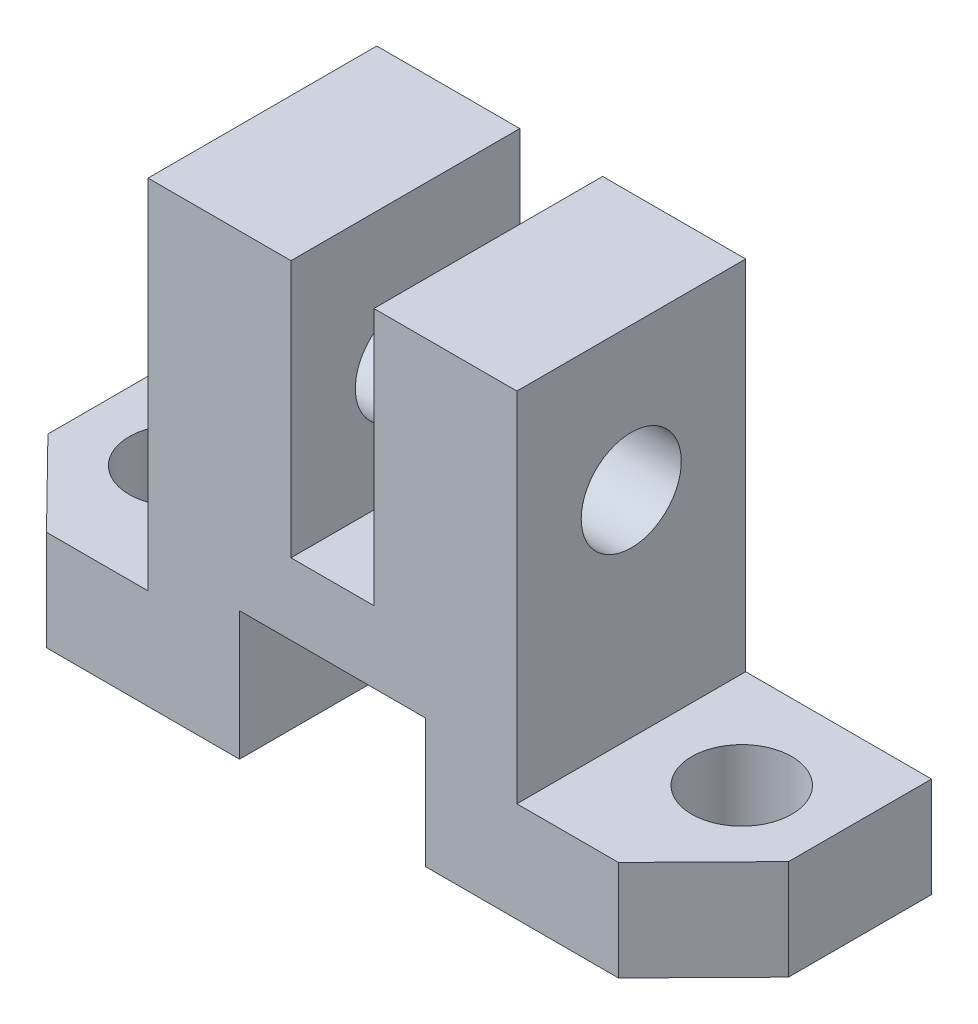
ISO-10303-21;
HEADER;
FILE_DESCRIPTION(('STEP AP214'),'2;1');
FILE_NAME('part.step','',(''),(''),'','','');
FILE_SCHEMA(('AUTOMOTIVE_DESIGN { 1 0 10303 214 1 1 1 1 }'));
ENDSEC;
DATA;
#1=APPLICATION_CONTEXT('core data for automotive mechanical design processes');
#2=APPLICATION_PROTOCOL_DEFINITION('international standard','automotive_design',2000,#1);
#3=PRODUCT_CONTEXT('',#1,'mechanical');
#4=PRODUCT('Part','Part','',(#3));
#5=PRODUCT_RELATED_PRODUCT_CATEGORY('part','',(#4));
#6=PRODUCT_DEFINITION_FORMATION('','',#4);
#7=PRODUCT_DEFINITION_CONTEXT('part definition',#1,'design');
#8=PRODUCT_DEFINITION('design','',#6,#7);
#9=PRODUCT_DEFINITION_SHAPE('','',#8);
#10=(LENGTH_UNIT() NAMED_UNIT(*) SI_UNIT(.MILLI.,.METRE.));
#11=(NAMED_UNIT(*) PLANE_ANGLE_UNIT() SI_UNIT($,.RADIAN.));
#12=(NAMED_UNIT(*) SI_UNIT($,.STERADIAN.) SOLID_ANGLE_UNIT());
#13=UNCERTAINTY_MEASURE_WITH_UNIT(LENGTH_MEASURE(1.E-05),#10,'distance_accuracy_value','');
#14=(GEOMETRIC_REPRESENTATION_CONTEXT(3) GLOBAL_UNCERTAINTY_ASSIGNED_CONTEXT((#13)) GLOBAL_UNIT_ASSIGNED_CONTEXT((#10,
#11,#12)) REPRESENTATION_CONTEXT('',''));
#15=CARTESIAN_POINT('',(0.,0.,0.));
#16=DIRECTION('',(0.,0.,1.));
#17=DIRECTION('',(1.,0.,0.));
#18=AXIS2_PLACEMENT_3D('',#15,#16,#17);
#19=CARTESIAN_POINT('',(-51.7969552583166,7.,2.19710608259383));
#20=DIRECTION('',(0.,0.,1.));
#21=DIRECTION('',(1.,0.,0.));
#22=AXIS2_PLACEMENT_3D('',#19,#20,#21);
#23=PLANE('',#22);
#24=DIRECTION('',(0.,-1.,0.));
#25=VECTOR('',#24,1.);
#26=CARTESIAN_POINT('',(-19.3984776291583,7.,2.19710608259383));
#27=LINE('',#26,#25);
#28=CARTESIAN_POINT('',(-19.3984776291583,9.,2.19710608259382));
#29=VERTEX_POINT('',#28);
#30=CARTESIAN_POINT('',(-19.3984776291583,0.,2.19710608259382));
#31=VERTEX_POINT('',#30);
#32=EDGE_CURVE('E190',#29,#31,#27,.T.);
#33=ORIENTED_EDGE('',*,*,#32,.F.);
#34=DIRECTION('',(1.,0.,0.));
#35=VECTOR('',#34,1.);
#36=CARTESIAN_POINT('',(-51.7969552583166,9.,2.19710608259383));
#37=LINE('',#36,#35);
#38=CARTESIAN_POINT('',(-32.3984776291583,9.,2.19710608259382));
#39=VERTEX_POINT('',#38);
#40=EDGE_CURVE('E186',#39,#29,#37,.T.);
#41=ORIENTED_EDGE('',*,*,#40,.F.);
#42=DIRECTION('',(0.,1.,0.));
#43=VECTOR('',#42,1.);
#44=CARTESIAN_POINT('',(-32.3984776291583,7.,2.19710608259383));
#45=LINE('',#44,#43);
#46=CARTESIAN_POINT('',(-32.3984776291583,0.,2.19710608259382));
#47=VERTEX_POINT('',#46);
#48=EDGE_CURVE('E172',#47,#39,#45,.T.);
#49=ORIENTED_EDGE('',*,*,#48,.F.);
#50=DIRECTION('',(-1.,0.,0.));
#51=VECTOR('',#50,1.);
#52=CARTESIAN_POINT('',(-51.7969552583166,0.,2.19710608259383));
#53=LINE('',#52,#51);
#54=CARTESIAN_POINT('',(-51.7969552583166,0.,2.19710608259383));
#55=VERTEX_POINT('',#54);
#56=EDGE_CURVE('E251',#47,#55,#53,.T.);
#57=ORIENTED_EDGE('',*,*,#56,.T.);
#58=DIRECTION('',(0.,-1.,0.));
#59=VECTOR('',#58,1.);
#60=CARTESIAN_POINT('',(-51.7969552583166,7.,2.19710608259383));
#61=LINE('',#60,#59);
#62=CARTESIAN_POINT('',(-51.7969552583166,7.,2.19710608259383));
#63=VERTEX_POINT('',#62);
#64=EDGE_CURVE('E298',#63,#55,#61,.T.);
#65=ORIENTED_EDGE('',*,*,#64,.F.);
#66=DIRECTION('',(-1.,0.,0.));
#67=VECTOR('',#66,1.);
#68=CARTESIAN_POINT('',(-51.7969552583166,7.,2.19710608259383));
#69=LINE('',#68,#67);
#70=CARTESIAN_POINT('',(-38.7969552583166,7.,2.19710608259383));
#71=VERTEX_POINT('',#70);
#72=EDGE_CURVE('E260',#71,#63,#69,.T.);
#73=ORIENTED_EDGE('',*,*,#72,.F.);
#74=DIRECTION('',(0.,-1.,0.));
#75=VECTOR('',#74,1.);
#76=CARTESIAN_POINT('',(-38.7969552583166,32.,2.19710608259383));
#77=LINE('',#76,#75);
#78=CARTESIAN_POINT('',(-38.7969552583166,32.,2.19710608259383));
#79=VERTEX_POINT('',#78);
#80=EDGE_CURVE('E240',#79,#71,#77,.T.);
#81=ORIENTED_EDGE('',*,*,#80,.F.);
#82=DIRECTION('',(-1.,0.,0.));
#83=VECTOR('',#82,1.);
#84=CARTESIAN_POINT('',(-38.7969552583166,32.,2.19710608259383));
#85=LINE('',#84,#83);
#86=CARTESIAN_POINT('',(-28.7969552583166,32.,2.19710608259382));
#87=VERTEX_POINT('',#86);
#88=EDGE_CURVE('E225',#87,#79,#85,.T.);
#89=ORIENTED_EDGE('',*,*,#88,.F.);
#90=DIRECTION('',(0.,1.,0.));
#91=VECTOR('',#90,1.);
#92=CARTESIAN_POINT('',(-28.7969552583166,7.,2.19710608259383));
#93=LINE('',#92,#91);
#94=CARTESIAN_POINT('',(-28.7969552583166,14.,2.19710608259382));
#95=VERTEX_POINT('',#94);
#96=EDGE_CURVE('E211',#95,#87,#93,.T.);
#97=ORIENTED_EDGE('',*,*,#96,.F.);
#98=DIRECTION('',(-1.,0.,0.));
#99=VECTOR('',#98,1.);
#100=CARTESIAN_POINT('',(-51.7969552583166,14.,2.19710608259383));
#101=LINE('',#100,#99);
#102=CARTESIAN_POINT('',(-23.,14.,2.19710608259382));
#103=VERTEX_POINT('',#102);
#104=EDGE_CURVE('E213',#103,#95,#101,.T.);
#105=ORIENTED_EDGE('',*,*,#104,.F.);
#106=DIRECTION('',(0.,-1.,0.));
#107=VECTOR('',#106,1.);
#108=CARTESIAN_POINT('',(-23.,7.00000000000001,2.19710608259383));
#109=LINE('',#108,#107);
#110=CARTESIAN_POINT('',(-23.,32.,2.19710608259382));
#111=VERTEX_POINT('',#110);
#112=EDGE_CURVE('E206',#111,#103,#109,.T.);
#113=ORIENTED_EDGE('',*,*,#112,.F.);
#114=CARTESIAN_POINT('',(-13.,32.,2.19710608259382));
#115=VERTEX_POINT('',#114);
#116=EDGE_CURVE('E223',#115,#111,#85,.T.);
#117=ORIENTED_EDGE('',*,*,#116,.F.);
#118=DIRECTION('',(0.,-1.,0.));
#119=VECTOR('',#118,1.);
#120=CARTESIAN_POINT('',(-13.,32.,2.19710608259382));
#121=LINE('',#120,#119);
#122=CARTESIAN_POINT('',(-13.,7.,2.19710608259382));
#123=VERTEX_POINT('',#122);
#124=EDGE_CURVE('E239',#115,#123,#121,.T.);
#125=ORIENTED_EDGE('',*,*,#124,.T.);
#126=CARTESIAN_POINT('',(0.,7.,2.19710608259383));
#127=VERTEX_POINT('',#126);
#128=EDGE_CURVE('E253',#127,#123,#69,.T.);
#129=ORIENTED_EDGE('',*,*,#128,.F.);
#130=DIRECTION('',(0.,-1.,0.));
#131=VECTOR('',#130,1.);
#132=CARTESIAN_POINT('',(0.,7.,2.19710608259383));
#133=LINE('',#132,#131);
#134=CARTESIAN_POINT('',(0.,0.,2.19710608259383));
#135=VERTEX_POINT('',#134);
#136=EDGE_CURVE('E268',#127,#135,#133,.T.);
#137=ORIENTED_EDGE('',*,*,#136,.T.);
#138=EDGE_CURVE('E267',#135,#31,#53,.T.);
#139=ORIENTED_EDGE('',*,*,#138,.T.);
#140=EDGE_LOOP('',(#33,#41,#49,#57,#65,#73,#81,#89,#97,#105,#113,#117,#125,#129,#137,#139));
#141=FACE_BOUND('',#140,.T.);
#142=ADVANCED_FACE('F39',(#141),#23,.F.);
#143=CARTESIAN_POINT('',(-45.8984776291583,7.,18.1971060825938));
#144=DIRECTION('',(0.,0.,-1.));
#145=DIRECTION('',(-1.,0.,0.));
#146=AXIS2_PLACEMENT_3D('',#143,#144,#145);
#147=PLANE('',#146);
#148=DIRECTION('',(0.,1.,0.));
#149=VECTOR('',#148,1.);
#150=CARTESIAN_POINT('',(-19.3984776291583,7.,18.1971060825938));
#151=LINE('',#150,#149);
#152=CARTESIAN_POINT('',(-19.3984776291583,0.,18.1971060825938));
#153=VERTEX_POINT('',#152);
#154=CARTESIAN_POINT('',(-19.3984776291583,9.,18.1971060825938));
#155=VERTEX_POINT('',#154);
#156=EDGE_CURVE('E185',#153,#155,#151,.T.);
#157=ORIENTED_EDGE('',*,*,#156,.F.);
#158=DIRECTION('',(1.,0.,0.));
#159=VECTOR('',#158,1.);
#160=CARTESIAN_POINT('',(-45.8984776291583,0.,18.1971060825938));
#161=LINE('',#160,#159);
#162=CARTESIAN_POINT('',(-5.89847762915829,0.,18.1971060825938));
#163=VERTEX_POINT('',#162);
#164=EDGE_CURVE('E276',#153,#163,#161,.T.);
#165=ORIENTED_EDGE('',*,*,#164,.T.);
#166=DIRECTION('',(0.,-1.,0.));
#167=VECTOR('',#166,1.);
#168=CARTESIAN_POINT('',(-5.89847762915829,7.,18.1971060825938));
#169=LINE('',#168,#167);
#170=CARTESIAN_POINT('',(-5.89847762915829,7.,18.1971060825938));
#171=VERTEX_POINT('',#170);
#172=EDGE_CURVE('E290',#171,#163,#169,.T.);
#173=ORIENTED_EDGE('',*,*,#172,.F.);
#174=DIRECTION('',(1.,0.,0.));
#175=VECTOR('',#174,1.);
#176=CARTESIAN_POINT('',(-45.8984776291583,7.,18.1971060825938));
#177=LINE('',#176,#175);
#178=CARTESIAN_POINT('',(-13.,7.,18.1971060825938));
#179=VERTEX_POINT('',#178);
#180=EDGE_CURVE('E265',#179,#171,#177,.T.);
#181=ORIENTED_EDGE('',*,*,#180,.F.);
#182=DIRECTION('',(0.,-1.,0.));
#183=VECTOR('',#182,1.);
#184=CARTESIAN_POINT('',(-13.,32.,18.1971060825938));
#185=LINE('',#184,#183);
#186=CARTESIAN_POINT('',(-13.,32.,18.1971060825938));
#187=VERTEX_POINT('',#186);
#188=EDGE_CURVE('E243',#187,#179,#185,.T.);
#189=ORIENTED_EDGE('',*,*,#188,.F.);
#190=DIRECTION('',(1.,0.,0.));
#191=VECTOR('',#190,1.);
#192=CARTESIAN_POINT('',(-13.,32.,18.1971060825938));
#193=LINE('',#192,#191);
#194=CARTESIAN_POINT('',(-23.,32.,18.1971060825938));
#195=VERTEX_POINT('',#194);
#196=EDGE_CURVE('E224',#195,#187,#193,.T.);
#197=ORIENTED_EDGE('',*,*,#196,.F.);
#198=DIRECTION('',(0.,1.,0.));
#199=VECTOR('',#198,1.);
#200=CARTESIAN_POINT('',(-23.,7.00000000000001,18.1971060825938));
#201=LINE('',#200,#199);
#202=CARTESIAN_POINT('',(-23.,14.,18.1971060825938));
#203=VERTEX_POINT('',#202);
#204=EDGE_CURVE('E64',#203,#195,#201,.T.);
#205=ORIENTED_EDGE('',*,*,#204,.F.);
#206=DIRECTION('',(1.,0.,0.));
#207=VECTOR('',#206,1.);
#208=CARTESIAN_POINT('',(-45.8984776291583,14.,18.1971060825938));
#209=LINE('',#208,#207);
#210=CARTESIAN_POINT('',(-28.7969552583166,14.,18.1971060825938));
#211=VERTEX_POINT('',#210);
#212=EDGE_CURVE('E310',#211,#203,#209,.T.);
#213=ORIENTED_EDGE('',*,*,#212,.F.);
#214=DIRECTION('',(0.,-1.,0.));
#215=VECTOR('',#214,1.);
#216=CARTESIAN_POINT('',(-28.7969552583166,7.,18.1971060825938));
#217=LINE('',#216,#215);
#218=CARTESIAN_POINT('',(-28.7969552583166,32.,18.1971060825938));
#219=VERTEX_POINT('',#218);
#220=EDGE_CURVE('E208',#219,#211,#217,.T.);
#221=ORIENTED_EDGE('',*,*,#220,.F.);
#222=CARTESIAN_POINT('',(-38.7969552583166,32.,18.1971060825938));
#223=VERTEX_POINT('',#222);
#224=EDGE_CURVE('E220',#223,#219,#193,.T.);
#225=ORIENTED_EDGE('',*,*,#224,.F.);
#226=DIRECTION('',(0.,-1.,0.));
#227=VECTOR('',#226,1.);
#228=CARTESIAN_POINT('',(-38.7969552583166,32.,18.1971060825938));
#229=LINE('',#228,#227);
#230=CARTESIAN_POINT('',(-38.7969552583166,7.,18.1971060825938));
#231=VERTEX_POINT('',#230);
#232=EDGE_CURVE('E230',#223,#231,#229,.T.);
#233=ORIENTED_EDGE('',*,*,#232,.T.);
#234=CARTESIAN_POINT('',(-45.8984776291583,7.,18.1971060825938));
#235=VERTEX_POINT('',#234);
#236=EDGE_CURVE('E264',#235,#231,#177,.T.);
#237=ORIENTED_EDGE('',*,*,#236,.F.);
#238=DIRECTION('',(0.,-1.,0.));
#239=VECTOR('',#238,1.);
#240=CARTESIAN_POINT('',(-45.8984776291583,7.,18.1971060825938));
#241=LINE('',#240,#239);
#242=CARTESIAN_POINT('',(-45.8984776291583,0.,18.1971060825938));
#243=VERTEX_POINT('',#242);
#244=EDGE_CURVE('E293',#235,#243,#241,.T.);
#245=ORIENTED_EDGE('',*,*,#244,.T.);
#246=CARTESIAN_POINT('',(-32.3984776291583,0.,18.1971060825938));
#247=VERTEX_POINT('',#246);
#248=EDGE_CURVE('E179',#243,#247,#161,.T.);
#249=ORIENTED_EDGE('',*,*,#248,.T.);
#250=DIRECTION('',(0.,-1.,0.));
#251=VECTOR('',#250,1.);
#252=CARTESIAN_POINT('',(-32.3984776291583,7.,18.1971060825938));
#253=LINE('',#252,#251);
#254=CARTESIAN_POINT('',(-32.3984776291583,9.,18.1971060825938));
#255=VERTEX_POINT('',#254);
#256=EDGE_CURVE('E52',#255,#247,#253,.T.);
#257=ORIENTED_EDGE('',*,*,#256,.F.);
#258=DIRECTION('',(-1.,0.,0.));
#259=VECTOR('',#258,1.);
#260=CARTESIAN_POINT('',(-45.8984776291583,9.,18.1971060825938));
#261=LINE('',#260,#259);
#262=EDGE_CURVE('E11',#155,#255,#261,.T.);
#263=ORIENTED_EDGE('',*,*,#262,.F.);
#264=EDGE_LOOP('',(#157,#165,#173,#181,#189,#197,#205,#213,#221,#225,#233,#237,#245,#249,#257,#263));
#265=FACE_BOUND('',#264,.T.);
#266=ADVANCED_FACE('F180',(#265),#147,.F.);
#267=CARTESIAN_POINT('',(0.,0.,0.));
#268=DIRECTION('',(0.,1.,0.));
#269=DIRECTION('',(0.,0.,1.));
#270=AXIS2_PLACEMENT_3D('',#267,#268,#269);
#271=PLANE('',#270);
#272=CARTESIAN_POINT('',(-6.25051200255727,0.,9.21864036847825));
#273=DIRECTION('',(0.,1.,0.));
#274=DIRECTION('',(0.,0.,1.));
#275=AXIS2_PLACEMENT_3D('',#272,#273,#274);
#276=CIRCLE('',#275,3.5);
#277=CARTESIAN_POINT('',(-6.25051200255727,0.,12.7186403684782));
#278=VERTEX_POINT('',#277);
#279=EDGE_CURVE('E246',#278,#278,#276,.F.);
#280=ORIENTED_EDGE('',*,*,#279,.F.);
#281=EDGE_LOOP('',(#280));
#282=FACE_BOUND('',#281,.T.);
#283=DIRECTION('',(0.,0.,1.));
#284=VECTOR('',#283,1.);
#285=CARTESIAN_POINT('',(-19.3984776291583,0.,0.));
#286=LINE('',#285,#284);
#287=EDGE_CURVE('E46',#31,#153,#286,.T.);
#288=ORIENTED_EDGE('',*,*,#287,.F.);
#289=ORIENTED_EDGE('',*,*,#138,.F.);
#290=DIRECTION('',(0.,0.,-1.));
#291=VECTOR('',#290,1.);
#292=CARTESIAN_POINT('',(0.,0.,12.1971060825938));
#293=LINE('',#292,#291);
#294=CARTESIAN_POINT('',(0.,0.,12.1971060825938));
#295=VERTEX_POINT('',#294);
#296=EDGE_CURVE('E282',#295,#135,#293,.T.);
#297=ORIENTED_EDGE('',*,*,#296,.F.);
#298=DIRECTION('',(0.701047956924281,0.,-0.713114129780284));
#299=VECTOR('',#298,1.);
#300=CARTESIAN_POINT('',(-5.89847762915829,0.,18.1971060825938));
#301=LINE('',#300,#299);
#302=EDGE_CURVE('E278',#163,#295,#301,.T.);
#303=ORIENTED_EDGE('',*,*,#302,.F.);
#304=ORIENTED_EDGE('',*,*,#164,.F.);
#305=EDGE_LOOP('',(#288,#289,#297,#303,#304));
#306=FACE_BOUND('',#305,.T.);
#307=ADVANCED_FACE('F324',(#282,#306),#271,.F.);
#308=CARTESIAN_POINT('',(-45.2969552583166,0.,9.51970674205226));
#309=DIRECTION('',(0.,1.,0.));
#310=DIRECTION('',(0.,0.,1.));
#311=AXIS2_PLACEMENT_3D('',#308,#309,#310);
#312=CIRCLE('',#311,3.5);
#313=CARTESIAN_POINT('',(-45.2969552583166,0.,13.0197067420523));
#314=VERTEX_POINT('',#313);
#315=EDGE_CURVE('E249',#314,#314,#312,.F.);
#316=ORIENTED_EDGE('',*,*,#315,.F.);
#317=EDGE_LOOP('',(#316));
#318=FACE_BOUND('',#317,.T.);
#319=DIRECTION('',(0.,0.,-1.));
#320=VECTOR('',#319,1.);
#321=CARTESIAN_POINT('',(-32.3984776291583,0.,0.));
#322=LINE('',#321,#320);
#323=EDGE_CURVE('E307',#247,#47,#322,.T.);
#324=ORIENTED_EDGE('',*,*,#323,.F.);
#325=ORIENTED_EDGE('',*,*,#248,.F.);
#326=DIRECTION('',(0.701047956924281,0.,0.713114129780284));
#327=VECTOR('',#326,1.);
#328=CARTESIAN_POINT('',(-45.8984776291583,0.,18.1971060825938));
#329=LINE('',#328,#327);
#330=CARTESIAN_POINT('',(-51.7969552583166,0.,12.1971060825938));
#331=VERTEX_POINT('',#330);
#332=EDGE_CURVE('E273',#331,#243,#329,.T.);
#333=ORIENTED_EDGE('',*,*,#332,.F.);
#334=DIRECTION('',(0.,0.,1.));
#335=VECTOR('',#334,1.);
#336=CARTESIAN_POINT('',(-51.7969552583166,0.,2.19710608259383));
#337=LINE('',#336,#335);
#338=EDGE_CURVE('E271',#55,#331,#337,.T.);
#339=ORIENTED_EDGE('',*,*,#338,.F.);
#340=ORIENTED_EDGE('',*,*,#56,.F.);
#341=EDGE_LOOP('',(#324,#325,#333,#339,#340));
#342=FACE_BOUND('',#341,.T.);
#343=ADVANCED_FACE('F385',(#318,#342),#271,.F.);
#344=CARTESIAN_POINT('',(0.,32.,0.));
#345=DIRECTION('',(0.,-1.,0.));
#346=DIRECTION('',(0.,0.,-1.));
#347=AXIS2_PLACEMENT_3D('',#344,#345,#346);
#348=PLANE('',#347);
#349=DIRECTION('',(0.,0.,1.));
#350=VECTOR('',#349,1.);
#351=CARTESIAN_POINT('',(-28.7969552583166,32.,0.));
#352=LINE('',#351,#350);
#353=EDGE_CURVE('E304',#87,#219,#352,.T.);
#354=ORIENTED_EDGE('',*,*,#353,.F.);
#355=ORIENTED_EDGE('',*,*,#88,.T.);
#356=DIRECTION('',(0.,0.,1.));
#357=VECTOR('',#356,1.);
#358=CARTESIAN_POINT('',(-38.7969552583166,32.,18.1971060825938));
#359=LINE('',#358,#357);
#360=EDGE_CURVE('E227',#79,#223,#359,.T.);
#361=ORIENTED_EDGE('',*,*,#360,.T.);
#362=ORIENTED_EDGE('',*,*,#224,.T.);
#363=EDGE_LOOP('',(#354,#355,#361,#362));
#364=FACE_BOUND('',#363,.T.);
#365=ADVANCED_FACE('F363',(#364),#348,.F.);
#366=DIRECTION('',(0.,0.,-1.));
#367=VECTOR('',#366,1.);
#368=CARTESIAN_POINT('',(-23.,32.,0.));
#369=LINE('',#368,#367);
#370=EDGE_CURVE('E299',#195,#111,#369,.T.);
#371=ORIENTED_EDGE('',*,*,#370,.F.);
#372=ORIENTED_EDGE('',*,*,#196,.T.);
#373=DIRECTION('',(0.,0.,-1.));
#374=VECTOR('',#373,1.);
#375=CARTESIAN_POINT('',(-13.,32.,2.19710608259382));
#376=LINE('',#375,#374);
#377=EDGE_CURVE('E218',#187,#115,#376,.T.);
#378=ORIENTED_EDGE('',*,*,#377,.T.);
#379=ORIENTED_EDGE('',*,*,#116,.T.);
#380=EDGE_LOOP('',(#371,#372,#378,#379));
#381=FACE_BOUND('',#380,.T.);
#382=ADVANCED_FACE('F343',(#381),#348,.F.);
#383=CARTESIAN_POINT('',(0.,7.,0.));
#384=DIRECTION('',(0.,1.,0.));
#385=DIRECTION('',(0.,0.,1.));
#386=AXIS2_PLACEMENT_3D('',#383,#384,#385);
#387=PLANE('',#386);
#388=DIRECTION('',(0.,0.,1.));
#389=VECTOR('',#388,1.);
#390=CARTESIAN_POINT('',(-38.7969552583166,7.,18.1971060825938));
#391=LINE('',#390,#389);
#392=EDGE_CURVE('E235',#71,#231,#391,.T.);
#393=ORIENTED_EDGE('',*,*,#392,.F.);
#394=ORIENTED_EDGE('',*,*,#72,.T.);
#395=DIRECTION('',(0.,0.,1.));
#396=VECTOR('',#395,1.);
#397=CARTESIAN_POINT('',(-51.7969552583166,7.,2.19710608259383));
#398=LINE('',#397,#396);
#399=CARTESIAN_POINT('',(-51.7969552583166,7.,12.1971060825938));
#400=VERTEX_POINT('',#399);
#401=EDGE_CURVE('E256',#63,#400,#398,.T.);
#402=ORIENTED_EDGE('',*,*,#401,.T.);
#403=DIRECTION('',(0.701047956924281,0.,0.713114129780284));
#404=VECTOR('',#403,1.);
#405=CARTESIAN_POINT('',(-45.8984776291583,7.,18.1971060825938));
#406=LINE('',#405,#404);
#407=EDGE_CURVE('E257',#400,#235,#406,.T.);
#408=ORIENTED_EDGE('',*,*,#407,.T.);
#409=ORIENTED_EDGE('',*,*,#236,.T.);
#410=EDGE_LOOP('',(#393,#394,#402,#408,#409));
#411=FACE_BOUND('',#410,.T.);
#412=CARTESIAN_POINT('',(-45.2969552583166,7.,9.51970674205226));
#413=DIRECTION('',(0.,1.,0.));
#414=DIRECTION('',(0.,0.,1.));
#415=AXIS2_PLACEMENT_3D('',#412,#413,#414);
#416=CIRCLE('',#415,3.5);
#417=CARTESIAN_POINT('',(-45.2969552583166,7.,13.0197067420523));
#418=VERTEX_POINT('',#417);
#419=EDGE_CURVE('E252',#418,#418,#416,.F.);
#420=ORIENTED_EDGE('',*,*,#419,.T.);
#421=EDGE_LOOP('',(#420));
#422=FACE_BOUND('',#421,.T.);
#423=ADVANCED_FACE('F375',(#411,#422),#387,.T.);
#424=CARTESIAN_POINT('',(-51.7969552583166,7.,2.19710608259383));
#425=DIRECTION('',(1.,0.,0.));
#426=DIRECTION('',(0.,0.,-1.));
#427=AXIS2_PLACEMENT_3D('',#424,#425,#426);
#428=PLANE('',#427);
#429=ORIENTED_EDGE('',*,*,#338,.T.);
#430=DIRECTION('',(0.,-1.,0.));
#431=VECTOR('',#430,1.);
#432=CARTESIAN_POINT('',(-51.7969552583166,7.,12.1971060825938));
#433=LINE('',#432,#431);
#434=EDGE_CURVE('E291',#400,#331,#433,.T.);
#435=ORIENTED_EDGE('',*,*,#434,.F.);
#436=ORIENTED_EDGE('',*,*,#401,.F.);
#437=ORIENTED_EDGE('',*,*,#64,.T.);
#438=EDGE_LOOP('',(#429,#435,#436,#437));
#439=FACE_BOUND('',#438,.T.);
#440=ADVANCED_FACE('F383',(#439),#428,.F.);
#441=CARTESIAN_POINT('',(-45.8984776291583,7.,18.1971060825938));
#442=DIRECTION('',(0.713114129780284,0.,-0.701047956924281));
#443=DIRECTION('',(-0.701047956924281,0.,-0.713114129780284));
#444=AXIS2_PLACEMENT_3D('',#441,#442,#443);
#445=PLANE('',#444);
#446=ORIENTED_EDGE('',*,*,#332,.T.);
#447=ORIENTED_EDGE('',*,*,#244,.F.);
#448=ORIENTED_EDGE('',*,*,#407,.F.);
#449=ORIENTED_EDGE('',*,*,#434,.T.);
#450=EDGE_LOOP('',(#446,#447,#448,#449));
#451=FACE_BOUND('',#450,.T.);
#452=ADVANCED_FACE('F377',(#451),#445,.F.);
#453=CARTESIAN_POINT('',(-5.89847762915829,7.,18.1971060825938));
#454=DIRECTION('',(-0.713114129780284,0.,-0.701047956924281));
#455=DIRECTION('',(-0.701047956924281,0.,0.713114129780284));
#456=AXIS2_PLACEMENT_3D('',#453,#454,#455);
#457=PLANE('',#456);
#458=ORIENTED_EDGE('',*,*,#302,.T.);
#459=DIRECTION('',(0.,-1.,0.));
#460=VECTOR('',#459,1.);
#461=CARTESIAN_POINT('',(0.,7.,12.1971060825938));
#462=LINE('',#461,#460);
#463=CARTESIAN_POINT('',(0.,7.,12.1971060825938));
#464=VERTEX_POINT('',#463);
#465=EDGE_CURVE('E283',#464,#295,#462,.T.);
#466=ORIENTED_EDGE('',*,*,#465,.F.);
#467=DIRECTION('',(0.701047956924281,0.,-0.713114129780284));
#468=VECTOR('',#467,1.);
#469=CARTESIAN_POINT('',(-5.89847762915829,7.,18.1971060825938));
#470=LINE('',#469,#468);
#471=EDGE_CURVE('E263',#171,#464,#470,.T.);
#472=ORIENTED_EDGE('',*,*,#471,.F.);
#473=ORIENTED_EDGE('',*,*,#172,.T.);
#474=EDGE_LOOP('',(#458,#466,#472,#473));
#475=FACE_BOUND('',#474,.T.);
#476=ADVANCED_FACE('F322',(#475),#457,.F.);
#477=CARTESIAN_POINT('',(0.,7.,12.1971060825938));
#478=DIRECTION('',(-1.,0.,0.));
#479=DIRECTION('',(0.,0.,1.));
#480=AXIS2_PLACEMENT_3D('',#477,#478,#479);
#481=PLANE('',#480);
#482=ORIENTED_EDGE('',*,*,#296,.T.);
#483=ORIENTED_EDGE('',*,*,#136,.F.);
#484=DIRECTION('',(0.,0.,-1.));
#485=VECTOR('',#484,1.);
#486=CARTESIAN_POINT('',(0.,7.,12.1971060825938));
#487=LINE('',#486,#485);
#488=EDGE_CURVE('E266',#464,#127,#487,.T.);
#489=ORIENTED_EDGE('',*,*,#488,.F.);
#490=ORIENTED_EDGE('',*,*,#465,.T.);
#491=EDGE_LOOP('',(#482,#483,#489,#490));
#492=FACE_BOUND('',#491,.T.);
#493=ADVANCED_FACE('F326',(#492),#481,.F.);
#494=DIRECTION('',(0.,0.,-1.));
#495=VECTOR('',#494,1.);
#496=CARTESIAN_POINT('',(-13.,7.,2.19710608259382));
#497=LINE('',#496,#495);
#498=EDGE_CURVE('E217',#179,#123,#497,.T.);
#499=ORIENTED_EDGE('',*,*,#498,.F.);
#500=ORIENTED_EDGE('',*,*,#180,.T.);
#501=ORIENTED_EDGE('',*,*,#471,.T.);
#502=ORIENTED_EDGE('',*,*,#488,.T.);
#503=ORIENTED_EDGE('',*,*,#128,.T.);
#504=EDGE_LOOP('',(#499,#500,#501,#502,#503));
#505=FACE_BOUND('',#504,.T.);
#506=CARTESIAN_POINT('',(-6.25051200255727,7.,9.21864036847825));
#507=DIRECTION('',(0.,1.,0.));
#508=DIRECTION('',(0.,0.,1.));
#509=AXIS2_PLACEMENT_3D('',#506,#507,#508);
#510=CIRCLE('',#509,3.5);
#511=CARTESIAN_POINT('',(-6.25051200255727,7.,12.7186403684782));
#512=VERTEX_POINT('',#511);
#513=EDGE_CURVE('E250',#512,#512,#510,.F.);
#514=ORIENTED_EDGE('',*,*,#513,.T.);
#515=EDGE_LOOP('',(#514));
#516=FACE_BOUND('',#515,.T.);
#517=ADVANCED_FACE('F335',(#505,#516),#387,.T.);
#518=CARTESIAN_POINT('',(-45.2969552583166,23.,9.51970674205226));
#519=DIRECTION('',(0.,-1.,0.));
#520=DIRECTION('',(0.,0.,-1.));
#521=AXIS2_PLACEMENT_3D('',#518,#519,#520);
#522=CYLINDRICAL_SURFACE('',#521,3.5);
#523=ORIENTED_EDGE('',*,*,#419,.F.);
#524=EDGE_LOOP('',(#523));
#525=FACE_BOUND('',#524,.T.);
#526=ORIENTED_EDGE('',*,*,#315,.T.);
#527=EDGE_LOOP('',(#526));
#528=FACE_BOUND('',#527,.T.);
#529=ADVANCED_FACE('F407',(#525,#528),#522,.F.);
#530=CARTESIAN_POINT('',(-6.25051200255727,34.,9.21864036847825));
#531=DIRECTION('',(0.,-1.,0.));
#532=DIRECTION('',(0.,0.,-1.));
#533=AXIS2_PLACEMENT_3D('',#530,#531,#532);
#534=CYLINDRICAL_SURFACE('',#533,3.5);
#535=ORIENTED_EDGE('',*,*,#513,.F.);
#536=EDGE_LOOP('',(#535));
#537=FACE_BOUND('',#536,.T.);
#538=ORIENTED_EDGE('',*,*,#279,.T.);
#539=EDGE_LOOP('',(#538));
#540=FACE_BOUND('',#539,.T.);
#541=ADVANCED_FACE('F414',(#537,#540),#534,.F.);
#542=CARTESIAN_POINT('',(-13.,32.,2.19710608259382));
#543=DIRECTION('',(-1.,0.,0.));
#544=DIRECTION('',(0.,0.,1.));
#545=AXIS2_PLACEMENT_3D('',#542,#543,#544);
#546=PLANE('',#545);
#547=CARTESIAN_POINT('',(-13.,22.,10.1971060825938));
#548=DIRECTION('',(-1.,0.,0.));
#549=DIRECTION('',(0.,0.,1.));
#550=AXIS2_PLACEMENT_3D('',#547,#548,#549);
#551=CIRCLE('',#550,3.5);
#552=CARTESIAN_POINT('',(-13.,22.,13.6971060825938));
#553=VERTEX_POINT('',#552);
#554=EDGE_CURVE('E199',#553,#553,#551,.T.);
#555=ORIENTED_EDGE('',*,*,#554,.T.);
#556=EDGE_LOOP('',(#555));
#557=FACE_BOUND('',#556,.T.);
#558=ORIENTED_EDGE('',*,*,#498,.T.);
#559=ORIENTED_EDGE('',*,*,#124,.F.);
#560=ORIENTED_EDGE('',*,*,#377,.F.);
#561=ORIENTED_EDGE('',*,*,#188,.T.);
#562=EDGE_LOOP('',(#558,#559,#560,#561));
#563=FACE_BOUND('',#562,.T.);
#564=ADVANCED_FACE('F338',(#557,#563),#546,.F.);
#565=CARTESIAN_POINT('',(-38.7969552583166,32.,18.1971060825938));
#566=DIRECTION('',(1.,0.,0.));
#567=DIRECTION('',(0.,0.,-1.));
#568=AXIS2_PLACEMENT_3D('',#565,#566,#567);
#569=PLANE('',#568);
#570=CARTESIAN_POINT('',(-38.7969552583166,22.,10.1971060825938));
#571=DIRECTION('',(1.,0.,0.));
#572=DIRECTION('',(0.,0.,-1.));
#573=AXIS2_PLACEMENT_3D('',#570,#571,#572);
#574=CIRCLE('',#573,3.5);
#575=CARTESIAN_POINT('',(-38.7969552583166,22.,6.69710608259383));
#576=VERTEX_POINT('',#575);
#577=EDGE_CURVE('E193',#576,#576,#574,.T.);
#578=ORIENTED_EDGE('',*,*,#577,.T.);
#579=EDGE_LOOP('',(#578));
#580=FACE_BOUND('',#579,.T.);
#581=ORIENTED_EDGE('',*,*,#392,.T.);
#582=ORIENTED_EDGE('',*,*,#232,.F.);
#583=ORIENTED_EDGE('',*,*,#360,.F.);
#584=ORIENTED_EDGE('',*,*,#80,.T.);
#585=EDGE_LOOP('',(#581,#582,#583,#584));
#586=FACE_BOUND('',#585,.T.);
#587=ADVANCED_FACE('F368',(#580,#586),#569,.F.);
#588=CARTESIAN_POINT('',(-23.,14.,56.1971060825938));
#589=DIRECTION('',(0.,1.,0.));
#590=DIRECTION('',(-1.,0.,0.));
#591=AXIS2_PLACEMENT_3D('',#588,#589,#590);
#592=PLANE('',#591);
#593=ORIENTED_EDGE('',*,*,#104,.T.);
#594=DIRECTION('',(0.,0.,-1.));
#595=VECTOR('',#594,1.);
#596=CARTESIAN_POINT('',(-28.7969552583166,14.,56.1971060825938));
#597=LINE('',#596,#595);
#598=EDGE_CURVE('E203',#211,#95,#597,.T.);
#599=ORIENTED_EDGE('',*,*,#598,.F.);
#600=ORIENTED_EDGE('',*,*,#212,.T.);
#601=DIRECTION('',(0.,0.,-1.));
#602=VECTOR('',#601,1.);
#603=CARTESIAN_POINT('',(-23.,14.,56.1971060825938));
#604=LINE('',#603,#602);
#605=EDGE_CURVE('E204',#203,#103,#604,.T.);
#606=ORIENTED_EDGE('',*,*,#605,.T.);
#607=EDGE_LOOP('',(#593,#599,#600,#606));
#608=FACE_BOUND('',#607,.T.);
#609=ADVANCED_FACE('F348',(#608),#592,.T.);
#610=CARTESIAN_POINT('',(-28.7969552583166,22.2471272516609,56.1971060825938));
#611=DIRECTION('',(1.,0.,0.));
#612=DIRECTION('',(0.,0.,-1.));
#613=AXIS2_PLACEMENT_3D('',#610,#611,#612);
#614=PLANE('',#613);
#615=CARTESIAN_POINT('',(-28.7969552583166,22.,10.1971060825938));
#616=DIRECTION('',(1.,0.,0.));
#617=DIRECTION('',(0.,0.,-1.));
#618=AXIS2_PLACEMENT_3D('',#615,#616,#617);
#619=CIRCLE('',#618,3.5);
#620=CARTESIAN_POINT('',(-28.7969552583166,22.,6.69710608259383));
#621=VERTEX_POINT('',#620);
#622=EDGE_CURVE('E194',#621,#621,#619,.T.);
#623=ORIENTED_EDGE('',*,*,#622,.F.);
#624=EDGE_LOOP('',(#623));
#625=FACE_BOUND('',#624,.T.);
#626=ORIENTED_EDGE('',*,*,#96,.T.);
#627=ORIENTED_EDGE('',*,*,#353,.T.);
#628=ORIENTED_EDGE('',*,*,#220,.T.);
#629=ORIENTED_EDGE('',*,*,#598,.T.);
#630=EDGE_LOOP('',(#626,#627,#628,#629));
#631=FACE_BOUND('',#630,.T.);
#632=ADVANCED_FACE('F356',(#625,#631),#614,.T.);
#633=CARTESIAN_POINT('',(-23.,32.,56.1971060825938));
#634=DIRECTION('',(-1.,0.,0.));
#635=DIRECTION('',(0.,-1.,0.));
#636=AXIS2_PLACEMENT_3D('',#633,#634,#635);
#637=PLANE('',#636);
#638=CARTESIAN_POINT('',(-23.,22.,10.1971060825938));
#639=DIRECTION('',(-1.,0.,0.));
#640=DIRECTION('',(0.,-1.,0.));
#641=AXIS2_PLACEMENT_3D('',#638,#639,#640);
#642=CIRCLE('',#641,3.5);
#643=CARTESIAN_POINT('',(-23.,18.5,10.1971060825938));
#644=VERTEX_POINT('',#643);
#645=EDGE_CURVE('E200',#644,#644,#642,.T.);
#646=ORIENTED_EDGE('',*,*,#645,.F.);
#647=EDGE_LOOP('',(#646));
#648=FACE_BOUND('',#647,.T.);
#649=ORIENTED_EDGE('',*,*,#112,.T.);
#650=ORIENTED_EDGE('',*,*,#605,.F.);
#651=ORIENTED_EDGE('',*,*,#204,.T.);
#652=ORIENTED_EDGE('',*,*,#370,.T.);
#653=EDGE_LOOP('',(#649,#650,#651,#652));
#654=FACE_BOUND('',#653,.T.);
#655=ADVANCED_FACE('F351',(#648,#654),#637,.T.);
#656=CARTESIAN_POINT('',(-26.,22.,10.1971060825938));
#657=DIRECTION('',(1.,0.,0.));
#658=DIRECTION('',(0.,0.,-1.));
#659=AXIS2_PLACEMENT_3D('',#656,#657,#658);
#660=CYLINDRICAL_SURFACE('',#659,3.5);
#661=ORIENTED_EDGE('',*,*,#645,.T.);
#662=EDGE_LOOP('',(#661));
#663=FACE_BOUND('',#662,.T.);
#664=ORIENTED_EDGE('',*,*,#554,.F.);
#665=EDGE_LOOP('',(#664));
#666=FACE_BOUND('',#665,.T.);
#667=ADVANCED_FACE('F433',(#663,#666),#660,.F.);
#668=CARTESIAN_POINT('',(-42.7969552583166,22.,10.1971060825938));
#669=DIRECTION('',(1.,0.,0.));
#670=DIRECTION('',(0.,0.,-1.));
#671=AXIS2_PLACEMENT_3D('',#668,#669,#670);
#672=CYLINDRICAL_SURFACE('',#671,3.5);
#673=ORIENTED_EDGE('',*,*,#622,.T.);
#674=EDGE_LOOP('',(#673));
#675=FACE_BOUND('',#674,.T.);
#676=ORIENTED_EDGE('',*,*,#577,.F.);
#677=EDGE_LOOP('',(#676));
#678=FACE_BOUND('',#677,.T.);
#679=ADVANCED_FACE('F440',(#675,#678),#672,.F.);
#680=CARTESIAN_POINT('',(-32.3984776291583,9.,35.1971060825938));
#681=DIRECTION('',(0.,-1.,0.));
#682=DIRECTION('',(0.,0.,-1.));
#683=AXIS2_PLACEMENT_3D('',#680,#681,#682);
#684=PLANE('',#683);
#685=ORIENTED_EDGE('',*,*,#40,.T.);
#686=DIRECTION('',(0.,0.,-1.));
#687=VECTOR('',#686,1.);
#688=CARTESIAN_POINT('',(-19.3984776291583,9.,35.1971060825938));
#689=LINE('',#688,#687);
#690=EDGE_CURVE('E169',#155,#29,#689,.T.);
#691=ORIENTED_EDGE('',*,*,#690,.F.);
#692=ORIENTED_EDGE('',*,*,#262,.T.);
#693=DIRECTION('',(0.,0.,-1.));
#694=VECTOR('',#693,1.);
#695=CARTESIAN_POINT('',(-32.3984776291583,9.,35.1971060825938));
#696=LINE('',#695,#694);
#697=EDGE_CURVE('E168',#255,#39,#696,.T.);
#698=ORIENTED_EDGE('',*,*,#697,.T.);
#699=EDGE_LOOP('',(#685,#691,#692,#698));
#700=FACE_BOUND('',#699,.T.);
#701=ADVANCED_FACE('F164',(#700),#684,.T.);
#702=CARTESIAN_POINT('',(-19.3984776291583,0.,35.1971060825938));
#703=DIRECTION('',(-1.,0.,0.));
#704=DIRECTION('',(0.,0.,1.));
#705=AXIS2_PLACEMENT_3D('',#702,#703,#704);
#706=PLANE('',#705);
#707=ORIENTED_EDGE('',*,*,#32,.T.);
#708=ORIENTED_EDGE('',*,*,#287,.T.);
#709=ORIENTED_EDGE('',*,*,#156,.T.);
#710=ORIENTED_EDGE('',*,*,#690,.T.);
#711=EDGE_LOOP('',(#707,#708,#709,#710));
#712=FACE_BOUND('',#711,.T.);
#713=ADVANCED_FACE('F313',(#712),#706,.T.);
#714=CARTESIAN_POINT('',(-32.3984776291583,0.,35.1971060825938));
#715=DIRECTION('',(1.,0.,0.));
#716=DIRECTION('',(0.,0.,-1.));
#717=AXIS2_PLACEMENT_3D('',#714,#715,#716);
#718=PLANE('',#717);
#719=ORIENTED_EDGE('',*,*,#48,.T.);
#720=ORIENTED_EDGE('',*,*,#697,.F.);
#721=ORIENTED_EDGE('',*,*,#256,.T.);
#722=ORIENTED_EDGE('',*,*,#323,.T.);
#723=EDGE_LOOP('',(#719,#720,#721,#722));
#724=FACE_BOUND('',#723,.T.);
#725=ADVANCED_FACE('F175',(#724),#718,.T.);
#726=CLOSED_SHELL('',(#142,#266,#307,#343,#365,#382,#423,#440,#452,#476,#493,#517,#529,#541,
#564,#587,#609,#632,#655,#667,#679,#701,#713,#725));
#727=MANIFOLD_SOLID_BREP('B2',#726);
#728=ADVANCED_BREP_SHAPE_REPRESENTATION('',(#18,#727),#14);
#729=SHAPE_DEFINITION_REPRESENTATION(#9,#728);
ENDSEC;
END-ISO-10303-21;
